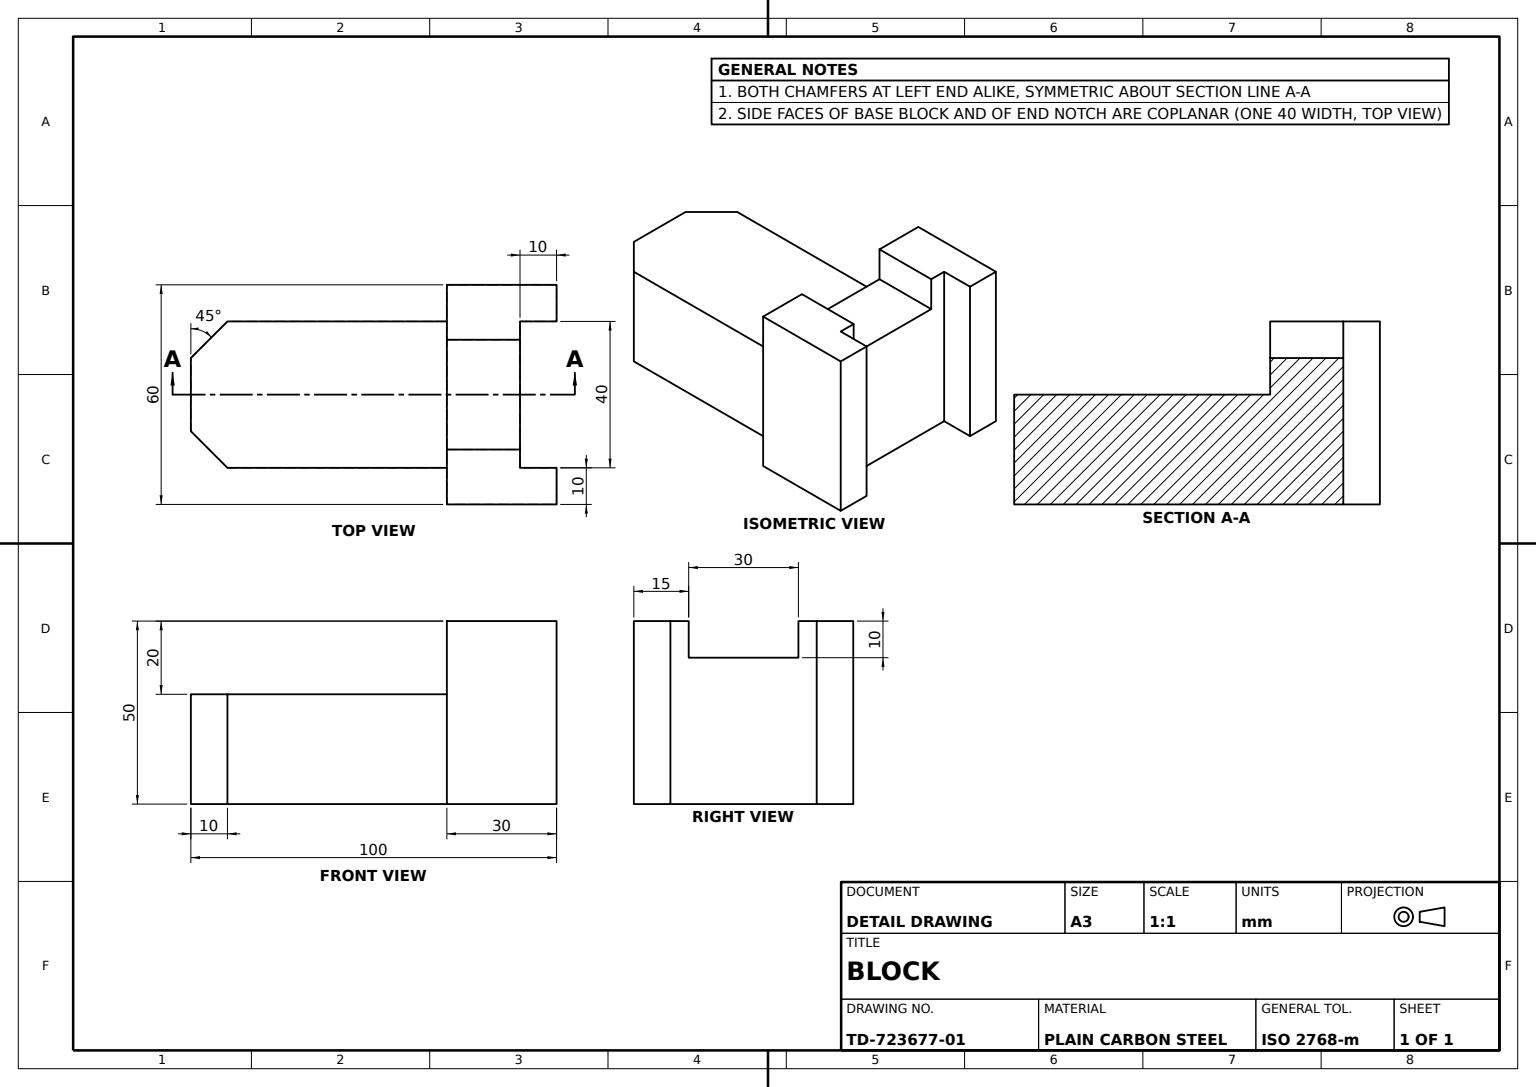
from build123d import *

# Parameters (mm, degrees)
CHAMFERED_BASE_BLOCK_DEPTH = 50
STEP_CUT_SKETCH_W          = 30
STEP_CUT_SKETCH_H          = 40
STEP_CUT_30X40_DEPTH       = 10
UPRIGHT_PROFILE_SKETCH_W   = 40
UPRIGHT_PROFILE_SKETCH_H   = 70
UPRIGHT_BLOCK_DEPTH        = 30
TOP_SLOT_CUT_DEPTH         = 30


with BuildPart() as part:
    # Base Profile Sketch → Chamfered Base Block (new body)
    with BuildSketch(Plane(origin=(0, 0, 0), x_dir=(1, 0, 0), z_dir=(0, 1, 0))):
        Polygon((0, 30), (0, 0), (60, 0), (60, 30), (50, 30), (50, 20), (26.160458453, 20), (10, 20), (10, 30), align=None)
    extrude(amount=CHAMFERED_BASE_BLOCK_DEPTH)

    # Step Cut Sketch → Step Cut 30x40 (cut)
    with BuildSketch(Plane(origin=(0, 50, 0), x_dir=(1, 0, 0), z_dir=(0, 1, 0))):
        with Locations((30, 0)):
            Rectangle(STEP_CUT_SKETCH_W, STEP_CUT_SKETCH_H)
    extrude(amount=-STEP_CUT_30X40_DEPTH, mode=Mode.SUBTRACT)

    # Upright Profile Sketch → Upright Block (add)
    with BuildSketch(Plane.XZ):
        with Locations((30, 35)):
            Rectangle(UPRIGHT_PROFILE_SKETCH_W, UPRIGHT_PROFILE_SKETCH_H)
    extrude(amount=-UPRIGHT_BLOCK_DEPTH)

    # Slot Sketch → Top Slot Cut (cut)
    with BuildSketch(Plane.XZ):
        Polygon((50, 60), (40, 70), (50, 70), align=None)
        Polygon((10, 70), (10, 60), (20, 70), align=None)
    extrude(amount=-TOP_SLOT_CUT_DEPTH, mode=Mode.SUBTRACT)


solid = part.part
